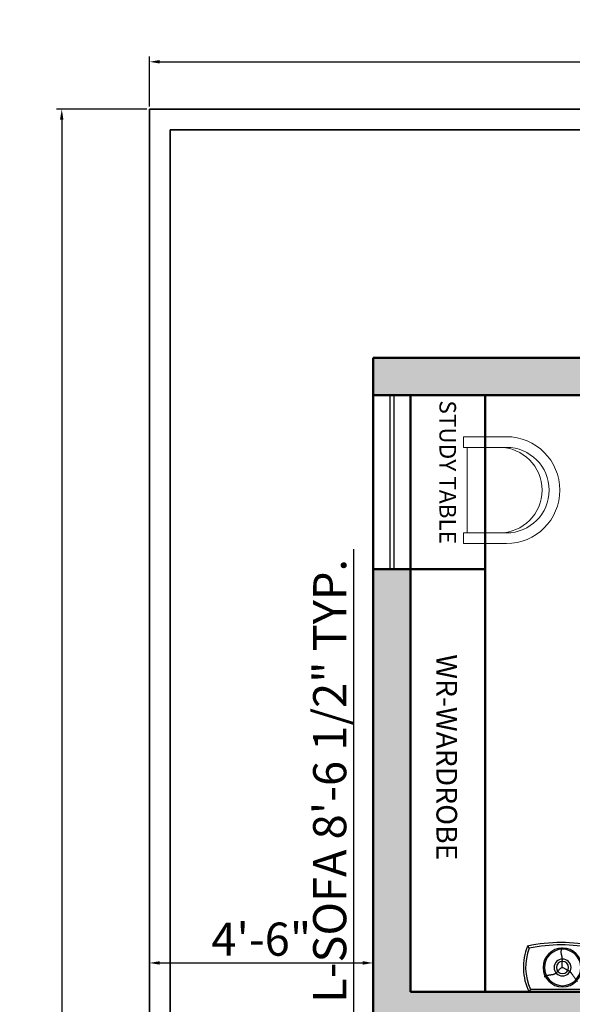
# Model space of a CAD drawing. Units: inches. Extents: x 3008 to 4088, y 1255 to 2137.
# Tile 26 of 30: x 3572 to 3705, y 1794 to 2031. Entities that reach past the tile are written whole.
import ezdxf

# ---------------------------------------------------------------- set-up
doc = ezdxf.new("R2010")
doc.units = ezdxf.units.IN
for name, color, linetype, lineweight in [('A-ANNO-DIMS', 2, 'Continuous', 18), ('A-ANNO-TEXT', 7, 'Continuous', 18), ('A-FURN', 8, 'Continuous', 18), ('A-GLAZ', 4, 'Continuous', 25), ('A-WALL', 7, 'Continuous', 50), ('A-WALL-PATT', 8, 'Continuous', 13), ('C-PROP', 1, 'Continuous', 35)]:
    doc.layers.add(name, color=color, linetype=linetype, lineweight=lineweight)
doc.layers.add('TEFRİŞ', color=11, linetype='Continuous')
doc.styles.get("Standard").update_dxf_attribs({"font": 'arial.ttf'})
doc.dimstyles.new('ISO-25', dxfattribs={"dimtxt": 8, "dimasz": 2.5, "dimexe": 1.25, "dimexo": 0.625, "dimtad": 1, "dimdec": 1, "dimlunit": 3, "dimtxsty": 'Standard', "dimcen": 2.5, "dimadec": 0, "dimazin": 0, "dimtfac": 1, "dimtdec": 1, "dimtmove": 0, "dimatfit": 3, "dimfxl": 1, "dimarcsym": 0})

# ---------------------------------------------------------------- blocks, each defined once
blk = doc.blocks.new('*D31')
at = {"layer": 'A-ANNO-DIMS', "color": 0, "lineweight": -2, "transparency": 16777216}
for p, q in [((3602.94, 2010.35), (3602.94, 2022.41)), ((4082.94, 2010.35), (4082.94, 2022.41)), ((3605.44, 2021.16), (4080.44, 2021.16))]:
    blk.add_line(p, q, dxfattribs=at)
at = {"layer": 'A-ANNO-DIMS', "color": 0, "transparency": 16777216}
for points in [[(3605.44, 2021.58), (3605.44, 2020.74), (3602.94, 2021.16)], [(4080.44, 2021.58), (4080.44, 2020.74), (4082.94, 2021.16)]]:
    blk.add_solid(points, dxfattribs=at)
at = {"layer": 'Defpoints', "color": 0, "transparency": 16777216}
for p in [(4082.94, 2021.16), (3602.94, 2009.72), (4082.94, 2009.72)]:
    blk.add_point(p, dxfattribs=at)
at = {"layer": 'A-ANNO-DIMS', "color": 0, "transparency": 16777216, "insert": (3842.94, 2025.87), "char_height": 8, "attachment_point": 5}
blk.add_mtext("40'", dxfattribs=at)
blk = doc.blocks.new('*D32')
at = {"layer": 'A-ANNO-DIMS', "color": 0, "lineweight": -2, "transparency": 16777216}
for p, q in [((3602.32, 2009.72), (3580.54, 2009.72)), ((3581.79, 2007.22), (3581.79, 1352.22)), ((3602.32, 1349.72), (3580.54, 1349.72))]:
    blk.add_line(p, q, dxfattribs=at)
at = {"layer": 'A-ANNO-DIMS', "color": 0, "transparency": 16777216}
for points in [[(3581.37, 2007.22), (3582.2, 2007.22), (3581.79, 2009.72)], [(3581.37, 1352.22), (3582.2, 1352.22), (3581.79, 1349.72)]]:
    blk.add_solid(points, dxfattribs=at)
at = {"layer": 'Defpoints', "color": 0, "transparency": 16777216}
for p in [(3602.94, 2009.72), (3581.79, 1349.72), (3602.94, 1349.72)]:
    blk.add_point(p, dxfattribs=at)
at = {"layer": 'A-ANNO-DIMS', "color": 0, "transparency": 16777216, "insert": (3577.09, 1679.72), "char_height": 8, "attachment_point": 5, "rotation": 90}
blk.add_mtext("55'", dxfattribs=at)
blk = doc.blocks.new('*D33')
at = {"layer": 'A-ANNO-DIMS', "color": 0, "lineweight": -2, "transparency": 16777216}
for p, q in [((3602.94, 1804.33), (3602.94, 1804.95)), ((3605.44, 1803.7), (3654.44, 1803.7)), ((3656.94, 1804.33), (3656.94, 1804.95))]:
    blk.add_line(p, q, dxfattribs=at)
at = {"layer": 'A-ANNO-DIMS', "color": 0, "transparency": 16777216}
for points in [[(3605.44, 1804.12), (3605.44, 1803.29), (3602.94, 1803.7)], [(3654.44, 1804.12), (3654.44, 1803.29), (3656.94, 1803.7)]]:
    blk.add_solid(points, dxfattribs=at)
at = {"layer": 'Defpoints', "color": 0, "transparency": 16777216}
for p in [(3602.94, 1803.7), (3656.94, 1803.7), (3656.94, 1803.7)]:
    blk.add_point(p, dxfattribs=at)
at = {"layer": 'A-ANNO-DIMS', "color": 0, "transparency": 16777216, "insert": (3629.94, 1808.41), "char_height": 8, "attachment_point": 5}
blk.add_mtext('4\'-6"', dxfattribs=at)
blk = doc.blocks.new('BED')
at = {"layer": 'TEFRİŞ'}
for p, q in [((2114.88, 1835.66), (2129.12, 1835.66)), ((2115.2, 1835.15), (2128.8, 1835.15)), ((2130.81, 1834.34), (2130.81, 1835.55)), ((2175.56, 1834.34), (2130.81, 1834.34)), ((2130.91, 1835.55), (2175.56, 1835.55)), ((2175, 1834.19), (2130.91, 1834.19)), ((2175.56, 1835.55), (2175.56, 1834.34)), ((2177.29, 1835.98), (2177.61, 1835.47)), ((2177.29, 1835.98), (2191.52, 1835.98)), ((2177.61, 1835.47), (2191.2, 1835.47)), ((2191.2, 1835.47), (2191.52, 1835.98)), ((2118.49, 1833.2), (2118.34, 1833.38)), ((2118.49, 1833.2), (2118.34, 1833.38)), ((2118.63, 1833.03), (2118.49, 1833.2)), ((2118.63, 1833.03), (2118.49, 1833.2)), ((2118.75, 1832.88), (2118.63, 1833.03)), ((2118.75, 1832.88), (2118.63, 1833.03)), ((2118.86, 1832.74), (2118.75, 1832.88)), ((2118.86, 1832.74), (2118.75, 1832.88)), ((2118.95, 1832.61), (2118.86, 1832.74)), ((2118.95, 1832.61), (2118.86, 1832.74)), ((2119.04, 1832.48), (2118.95, 1832.61)), ((2119.04, 1832.48), (2118.95, 1832.61)), ((2119.12, 1832.37), (2119.04, 1832.48)), ((2119.12, 1832.37), (2119.04, 1832.48)), ((2119.19, 1832.26), (2119.12, 1832.37)), ((2119.19, 1832.26), (2119.12, 1832.37)), ((2119.26, 1832.16), (2119.19, 1832.26)), ((2119.26, 1832.16), (2119.19, 1832.26)), ((2119.32, 1832.06), (2119.26, 1832.16)), ((2119.32, 1832.06), (2119.26, 1832.16)), ((2119.39, 1831.97), (2119.32, 1832.06)), ((2119.39, 1831.97), (2119.32, 1832.06)), ((2119.45, 1831.89), (2119.39, 1831.97)), ((2119.45, 1831.89), (2119.39, 1831.97)), ((2124.49, 1831.94), (2124.56, 1831.95)), ((2124.49, 1831.94), (2124.56, 1831.95)), ((2124.56, 1831.95), (2124.64, 1831.96)), ((2124.56, 1831.95), (2124.64, 1831.96)), ((2124.64, 1831.96), (2124.71, 1831.98)), ((2124.64, 1831.96), (2124.71, 1831.98)), ((2124.71, 1831.98), (2124.79, 1831.99)), ((2124.71, 1831.98), (2124.79, 1831.99)), ((2124.79, 1831.99), (2124.87, 1832.01)), ((2124.79, 1831.99), (2124.87, 1832.01)), ((2124.87, 1832.01), (2124.96, 1832.03)), ((2124.87, 1832.01), (2124.96, 1832.03)), ((2124.96, 1832.03), (2125.05, 1832.05)), ((2124.96, 1832.03), (2125.05, 1832.05)), ((2125.05, 1832.05), (2125.14, 1832.08)), ((2125.05, 1832.05), (2125.14, 1832.08)), ((2125.14, 1832.08), (2125.23, 1832.11)), ((2125.14, 1832.08), (2125.23, 1832.11)), ((2125.23, 1832.11), (2125.33, 1832.14)), ((2125.23, 1832.11), (2125.33, 1832.14)), ((2125.33, 1832.14), (2125.42, 1832.17)), ((2125.33, 1832.14), (2125.42, 1832.17)), ((2125.42, 1832.17), (2125.52, 1832.21)), ((2125.42, 1832.17), (2125.52, 1832.21)), ((2125.52, 1832.21), (2125.6, 1832.25)), ((2125.52, 1832.21), (2125.6, 1832.25)), ((2125.6, 1832.25), (2125.68, 1832.3)), ((2125.6, 1832.25), (2125.68, 1832.3)), ((2125.68, 1832.3), (2125.75, 1832.35)), ((2125.68, 1832.3), (2125.75, 1832.35)), ((2180.9, 1833.52), (2180.75, 1833.7)), ((2180.9, 1833.52), (2180.75, 1833.7)), ((2181.04, 1833.35), (2180.9, 1833.52)), ((2181.04, 1833.35), (2180.9, 1833.52)), ((2181.16, 1833.2), (2181.04, 1833.35)), ((2181.16, 1833.2), (2181.04, 1833.35)), ((2181.26, 1833.06), (2181.16, 1833.2)), ((2181.26, 1833.06), (2181.16, 1833.2)), ((2181.36, 1832.93), (2181.26, 1833.06)), ((2181.36, 1832.93), (2181.26, 1833.06)), ((2181.44, 1832.8), (2181.36, 1832.93)), ((2181.44, 1832.8), (2181.36, 1832.93)), ((2181.52, 1832.69), (2181.44, 1832.8)), ((2181.52, 1832.69), (2181.44, 1832.8)), ((2181.59, 1832.58), (2181.52, 1832.69)), ((2181.59, 1832.58), (2181.52, 1832.69)), ((2181.66, 1832.48), (2181.59, 1832.58)), ((2181.66, 1832.48), (2181.59, 1832.58)), ((2181.73, 1832.38), (2181.66, 1832.48)), ((2181.73, 1832.38), (2181.66, 1832.48)), ((2181.79, 1832.29), (2181.73, 1832.38)), ((2181.79, 1832.29), (2181.73, 1832.38)), ((2181.85, 1832.21), (2181.79, 1832.29)), ((2181.85, 1832.21), (2181.79, 1832.29)), ((2181.92, 1832.13), (2181.85, 1832.21)), ((2181.92, 1832.13), (2181.85, 1832.21)), ((2181.97, 1832.05), (2181.92, 1832.13)), ((2181.97, 1832.05), (2181.92, 1832.13)), ((2182.03, 1831.97), (2181.97, 1832.05)), ((2182.03, 1831.97), (2181.97, 1832.05)), ((2182.09, 1831.9), (2182.03, 1831.97)), ((2182.09, 1831.9), (2182.03, 1831.97)), ((2185.68, 1831.9), (2185.75, 1831.95)), ((2185.68, 1831.9), (2185.75, 1831.95)), ((2185.75, 1831.95), (2185.82, 1831.99)), ((2185.75, 1831.95), (2185.82, 1831.99)), ((2185.82, 1831.99), (2185.89, 1832.03)), ((2185.82, 1831.99), (2185.89, 1832.03)), ((2185.89, 1832.03), (2185.96, 1832.06)), ((2185.89, 1832.03), (2185.96, 1832.06)), ((2185.96, 1832.06), (2186.03, 1832.09)), ((2185.96, 1832.06), (2186.03, 1832.09)), ((2186.03, 1832.09), (2186.1, 1832.12)), ((2186.03, 1832.09), (2186.1, 1832.12)), ((2186.1, 1832.12), (2186.17, 1832.14)), ((2186.1, 1832.12), (2186.17, 1832.14)), ((2186.17, 1832.14), (2186.24, 1832.16)), ((2186.17, 1832.14), (2186.24, 1832.16)), ((2186.24, 1832.16), (2186.32, 1832.18)), ((2186.24, 1832.16), (2186.32, 1832.18)), ((2186.32, 1832.18), (2186.39, 1832.19)), ((2186.32, 1832.18), (2186.39, 1832.19)), ((2186.39, 1832.19), (2186.46, 1832.21)), ((2186.39, 1832.19), (2186.46, 1832.21)), ((2186.46, 1832.21), (2186.53, 1832.22)), ((2186.46, 1832.21), (2186.53, 1832.22)), ((2186.53, 1832.22), (2186.61, 1832.23)), ((2186.53, 1832.22), (2186.61, 1832.23)), ((2186.61, 1832.23), (2186.68, 1832.23)), ((2186.61, 1832.23), (2186.68, 1832.23)), ((2186.68, 1832.23), (2186.75, 1832.24)), ((2186.68, 1832.23), (2186.75, 1832.24)), ((2186.75, 1832.24), (2186.82, 1832.25)), ((2186.75, 1832.24), (2186.82, 1832.25)), ((2186.82, 1832.25), (2186.9, 1832.26)), ((2186.82, 1832.25), (2186.9, 1832.26)), ((2186.9, 1832.26), (2186.97, 1832.27)), ((2186.9, 1832.26), (2186.97, 1832.27)), ((2186.97, 1832.27), (2187.04, 1832.28)), ((2186.97, 1832.27), (2187.04, 1832.28)), ((2187.04, 1832.28), (2187.12, 1832.3)), ((2187.04, 1832.28), (2187.12, 1832.3)), ((2187.12, 1832.3), (2187.2, 1832.31)), ((2187.12, 1832.3), (2187.2, 1832.31)), ((2187.2, 1832.31), (2187.28, 1832.33)), ((2187.2, 1832.31), (2187.28, 1832.33)), ((2187.28, 1832.33), (2187.36, 1832.35)), ((2187.28, 1832.33), (2187.36, 1832.35)), ((2187.36, 1832.35), (2187.45, 1832.37)), ((2187.36, 1832.35), (2187.45, 1832.37)), ((2187.45, 1832.37), (2187.54, 1832.4)), ((2187.45, 1832.37), (2187.54, 1832.4)), ((2187.54, 1832.4), (2187.64, 1832.43)), ((2187.54, 1832.4), (2187.64, 1832.43)), ((2187.64, 1832.43), (2187.74, 1832.46)), ((2187.64, 1832.43), (2187.74, 1832.46)), ((2187.74, 1832.46), (2187.83, 1832.49)), ((2187.74, 1832.46), (2187.83, 1832.49)), ((2187.83, 1832.49), (2187.92, 1832.53)), ((2187.83, 1832.49), (2187.92, 1832.53)), ((2187.92, 1832.53), (2188.01, 1832.57)), ((2187.92, 1832.53), (2188.01, 1832.57)), ((2188.01, 1832.57), (2188.09, 1832.62)), ((2188.01, 1832.57), (2188.09, 1832.62)), ((2188.09, 1832.62), (2188.15, 1832.67)), ((2188.09, 1832.62), (2188.15, 1832.67)), ((2119.51, 1831.81), (2119.45, 1831.89)), ((2119.51, 1831.81), (2119.45, 1831.89)), ((2119.57, 1831.73), (2119.51, 1831.81)), ((2119.57, 1831.73), (2119.51, 1831.81)), ((2119.63, 1831.65), (2119.57, 1831.73)), ((2119.63, 1831.65), (2119.57, 1831.73)), ((2119.69, 1831.58), (2119.63, 1831.65)), ((2119.69, 1831.58), (2119.63, 1831.65)), ((2119.75, 1831.51), (2119.69, 1831.58)), ((2119.75, 1831.51), (2119.69, 1831.58)), ((2119.81, 1831.44), (2119.75, 1831.51)), ((2119.81, 1831.44), (2119.75, 1831.51)), ((2119.87, 1831.38), (2119.81, 1831.44)), ((2119.87, 1831.38), (2119.81, 1831.44)), ((2119.93, 1831.31), (2119.87, 1831.38)), ((2119.93, 1831.31), (2119.87, 1831.38)), ((2119.99, 1831.25), (2119.93, 1831.31)), ((2119.99, 1831.25), (2119.93, 1831.31)), ((2120.05, 1831.2), (2119.99, 1831.25)), ((2120.05, 1831.2), (2119.99, 1831.25)), ((2120.12, 1831.14), (2120.05, 1831.2)), ((2120.12, 1831.14), (2120.05, 1831.2)), ((2120.18, 1831.09), (2120.12, 1831.14)), ((2120.18, 1831.09), (2120.12, 1831.14)), ((2120.25, 1831.04), (2120.18, 1831.09)), ((2120.25, 1831.04), (2120.18, 1831.09)), ((2120.32, 1830.99), (2120.25, 1831.04)), ((2120.32, 1830.99), (2120.25, 1831.04)), ((2120.39, 1830.94), (2120.32, 1830.99)), ((2120.39, 1830.94), (2120.32, 1830.99)), ((2120.47, 1830.9), (2120.39, 1830.94)), ((2120.47, 1830.9), (2120.39, 1830.94)), ((2120.54, 1830.85), (2120.47, 1830.9)), ((2120.54, 1830.85), (2120.47, 1830.9)), ((2120.62, 1830.8), (2120.54, 1830.85)), ((2120.62, 1830.8), (2120.54, 1830.85)), ((2120.7, 1830.75), (2120.62, 1830.8)), ((2120.7, 1830.75), (2120.62, 1830.8)), ((2120.79, 1830.7), (2120.7, 1830.75)), ((2120.79, 1830.7), (2120.7, 1830.75)), ((2120.88, 1830.65), (2120.79, 1830.7)), ((2120.88, 1830.65), (2120.79, 1830.7)), ((2120.98, 1830.59), (2120.88, 1830.65)), ((2120.98, 1830.59), (2120.88, 1830.65)), ((2121.09, 1830.52), (2120.98, 1830.59)), ((2121.09, 1830.52), (2120.98, 1830.59)), ((2121.21, 1830.45), (2121.09, 1830.52)), ((2121.21, 1830.45), (2121.09, 1830.52)), ((2121.34, 1830.38), (2121.21, 1830.45)), ((2121.34, 1830.38), (2121.21, 1830.45)), ((2121.49, 1830.29), (2121.34, 1830.38)), ((2121.49, 1830.29), (2121.34, 1830.38)), ((2121.66, 1830.21), (2121.49, 1830.29)), ((2121.66, 1830.21), (2121.49, 1830.29)), ((2121.66, 1830.18), (2121.87, 1830.29)), ((2121.66, 1830.18), (2121.87, 1830.29)), ((2121.85, 1830.11), (2121.66, 1830.21)), ((2121.85, 1830.11), (2121.66, 1830.21)), ((2121.74, 1829.99), (2121.73, 1829.83)), ((2121.74, 1829.99), (2121.73, 1829.83)), ((2121.73, 1829.83), (2121.73, 1829.69)), ((2121.73, 1829.83), (2121.73, 1829.69)), ((2121.76, 1830.38), (2121.74, 1830.17)), ((2121.76, 1830.38), (2121.74, 1830.17)), ((2121.74, 1830.17), (2121.74, 1829.99)), ((2121.74, 1830.17), (2121.74, 1829.99)), ((2121.87, 1830.29), (2122.04, 1830.4)), ((2121.87, 1830.29), (2122.04, 1830.4)), ((2122.04, 1830.4), (2122.2, 1830.51)), ((2122.04, 1830.4), (2122.2, 1830.51)), ((2122.2, 1830.51), (2122.33, 1830.61)), ((2122.2, 1830.51), (2122.33, 1830.61)), ((2122.33, 1830.61), (2122.45, 1830.72)), ((2122.33, 1830.61), (2122.45, 1830.72)), ((2122.45, 1830.72), (2122.55, 1830.82)), ((2122.45, 1830.72), (2122.55, 1830.82)), ((2122.55, 1830.82), (2122.64, 1830.91)), ((2122.55, 1830.82), (2122.64, 1830.91)), ((2122.64, 1830.91), (2122.72, 1831.01)), ((2122.64, 1830.91), (2122.72, 1831.01)), ((2122.72, 1831.01), (2122.8, 1831.09)), ((2122.72, 1831.01), (2122.8, 1831.09)), ((2122.8, 1831.09), (2122.87, 1831.18)), ((2122.8, 1831.09), (2122.87, 1831.18)), ((2122.87, 1831.18), (2122.94, 1831.26)), ((2122.87, 1831.18), (2122.94, 1831.26)), ((2122.94, 1831.26), (2123.01, 1831.33)), ((2122.94, 1831.26), (2123.01, 1831.33)), ((2123.01, 1831.33), (2123.08, 1831.4)), ((2123.01, 1831.33), (2123.08, 1831.4)), ((2123.08, 1831.4), (2123.14, 1831.46)), ((2123.08, 1831.4), (2123.14, 1831.46)), ((2123.14, 1831.46), (2123.21, 1831.52)), ((2123.14, 1831.46), (2123.21, 1831.52)), ((2123.21, 1831.52), (2123.27, 1831.58)), ((2123.21, 1831.52), (2123.27, 1831.58)), ((2123.27, 1831.58), (2123.34, 1831.63)), ((2123.27, 1831.58), (2123.34, 1831.63)), ((2123.34, 1831.63), (2123.41, 1831.67)), ((2123.34, 1831.63), (2123.41, 1831.67)), ((2123.41, 1831.67), (2123.48, 1831.71)), ((2123.41, 1831.67), (2123.48, 1831.71)), ((2123.48, 1831.71), (2123.55, 1831.74)), ((2123.48, 1831.71), (2123.55, 1831.74)), ((2123.55, 1831.74), (2123.62, 1831.77)), ((2123.55, 1831.74), (2123.62, 1831.77)), ((2123.62, 1831.77), (2123.69, 1831.8)), ((2123.62, 1831.77), (2123.69, 1831.8)), ((2123.69, 1831.8), (2123.77, 1831.82)), ((2123.69, 1831.8), (2123.77, 1831.82)), ((2123.77, 1831.82), (2123.84, 1831.84)), ((2123.77, 1831.82), (2123.84, 1831.84)), ((2123.84, 1831.84), (2123.91, 1831.86)), ((2123.84, 1831.84), (2123.91, 1831.86)), ((2123.91, 1831.86), (2123.98, 1831.87)), ((2123.91, 1831.86), (2123.98, 1831.87)), ((2123.98, 1831.87), (2124.06, 1831.89)), ((2123.98, 1831.87), (2124.06, 1831.89)), ((2124.06, 1831.89), (2124.13, 1831.9)), ((2124.06, 1831.89), (2124.13, 1831.9)), ((2124.13, 1831.9), (2124.2, 1831.91)), ((2124.13, 1831.9), (2124.2, 1831.91)), ((2124.2, 1831.91), (2124.27, 1831.91)), ((2124.2, 1831.91), (2124.27, 1831.91)), ((2124.27, 1831.91), (2124.35, 1831.92)), ((2124.27, 1831.91), (2124.35, 1831.92)), ((2124.35, 1831.92), (2124.42, 1831.93)), ((2124.35, 1831.92), (2124.42, 1831.93)), ((2124.42, 1831.93), (2124.49, 1831.94)), ((2124.42, 1831.93), (2124.49, 1831.94)), ((2182.15, 1831.83), (2182.09, 1831.9)), ((2182.15, 1831.83), (2182.09, 1831.9)), ((2182.21, 1831.76), (2182.15, 1831.83)), ((2182.21, 1831.76), (2182.15, 1831.83)), ((2182.27, 1831.7), (2182.21, 1831.76)), ((2182.27, 1831.7), (2182.21, 1831.76)), ((2182.33, 1831.63), (2182.27, 1831.7)), ((2182.33, 1831.63), (2182.27, 1831.7)), ((2182.4, 1831.57), (2182.33, 1831.63)), ((2182.4, 1831.57), (2182.33, 1831.63)), ((2182.46, 1831.52), (2182.4, 1831.57)), ((2182.46, 1831.52), (2182.4, 1831.57)), ((2182.52, 1831.46), (2182.46, 1831.52)), ((2182.52, 1831.46), (2182.46, 1831.52)), ((2182.59, 1831.41), (2182.52, 1831.46)), ((2182.59, 1831.41), (2182.52, 1831.46)), ((2182.66, 1831.36), (2182.59, 1831.41)), ((2182.66, 1831.36), (2182.59, 1831.41)), ((2182.73, 1831.31), (2182.66, 1831.36)), ((2182.73, 1831.31), (2182.66, 1831.36)), ((2182.8, 1831.26), (2182.73, 1831.31)), ((2182.8, 1831.26), (2182.73, 1831.31)), ((2182.87, 1831.22), (2182.8, 1831.26)), ((2182.87, 1831.22), (2182.8, 1831.26)), ((2182.95, 1831.17), (2182.87, 1831.22)), ((2182.95, 1831.17), (2182.87, 1831.22)), ((2183.03, 1831.12), (2182.95, 1831.17)), ((2183.03, 1831.12), (2182.95, 1831.17)), ((2183.11, 1831.07), (2183.03, 1831.12)), ((2183.11, 1831.07), (2183.03, 1831.12)), ((2183.2, 1831.02), (2183.11, 1831.07)), ((2183.2, 1831.02), (2183.11, 1831.07)), ((2183.29, 1830.97), (2183.2, 1831.02)), ((2183.29, 1830.97), (2183.2, 1831.02)), ((2183.39, 1830.91), (2183.29, 1830.97)), ((2183.39, 1830.91), (2183.29, 1830.97)), ((2183.49, 1830.84), (2183.39, 1830.91)), ((2183.49, 1830.84), (2183.39, 1830.91)), ((2183.61, 1830.77), (2183.49, 1830.84)), ((2183.61, 1830.77), (2183.49, 1830.84)), ((2183.75, 1830.7), (2183.61, 1830.77)), ((2183.75, 1830.7), (2183.61, 1830.77)), ((2183.9, 1830.61), (2183.75, 1830.7)), ((2183.9, 1830.61), (2183.75, 1830.7)), ((2184.06, 1830.53), (2183.9, 1830.61)), ((2184.06, 1830.53), (2183.9, 1830.61)), ((2184.25, 1830.43), (2184.06, 1830.53)), ((2184.25, 1830.43), (2184.06, 1830.53)), ((2184.07, 1830.5), (2184.27, 1830.61)), ((2184.07, 1830.5), (2184.27, 1830.61)), ((2184.15, 1830.49), (2184.14, 1830.31)), ((2184.15, 1830.49), (2184.14, 1830.31)), ((2184.14, 1830.31), (2184.14, 1830.15)), ((2184.14, 1830.31), (2184.14, 1830.15)), ((2184.14, 1830.15), (2184.14, 1830.01)), ((2184.14, 1830.15), (2184.14, 1830.01)), ((2184.14, 1830.01), (2184.14, 1829.89)), ((2184.14, 1830.01), (2184.14, 1829.89)), ((2184.14, 1829.89), (2184.14, 1829.77)), ((2184.14, 1829.89), (2184.14, 1829.77)), ((2184.14, 1829.77), (2184.14, 1829.67)), ((2184.14, 1829.77), (2184.14, 1829.67)), ((2184.17, 1830.7), (2184.15, 1830.49)), ((2184.17, 1830.7), (2184.15, 1830.49)), ((2184.27, 1830.61), (2184.45, 1830.72)), ((2184.27, 1830.61), (2184.45, 1830.72)), ((2184.45, 1830.72), (2184.6, 1830.83)), ((2184.45, 1830.72), (2184.6, 1830.83)), ((2184.6, 1830.83), (2184.74, 1830.93)), ((2184.6, 1830.83), (2184.74, 1830.93)), ((2184.74, 1830.93), (2184.85, 1831.04)), ((2184.74, 1830.93), (2184.85, 1831.04)), ((2184.85, 1831.04), (2184.95, 1831.14)), ((2184.85, 1831.04), (2184.95, 1831.14)), ((2184.95, 1831.14), (2185.05, 1831.23)), ((2184.95, 1831.14), (2185.05, 1831.23)), ((2185.05, 1831.23), (2185.13, 1831.33)), ((2185.05, 1831.23), (2185.13, 1831.33)), ((2185.13, 1831.33), (2185.21, 1831.41)), ((2185.13, 1831.33), (2185.21, 1831.41)), ((2185.21, 1831.41), (2185.28, 1831.5)), ((2185.21, 1831.41), (2185.28, 1831.5)), ((2185.28, 1831.5), (2185.35, 1831.58)), ((2185.28, 1831.5), (2185.35, 1831.58)), ((2185.35, 1831.58), (2185.42, 1831.65)), ((2185.35, 1831.58), (2185.42, 1831.65)), ((2185.42, 1831.65), (2185.48, 1831.72)), ((2185.42, 1831.65), (2185.48, 1831.72)), ((2185.48, 1831.72), (2185.55, 1831.78)), ((2185.48, 1831.72), (2185.55, 1831.78)), ((2185.55, 1831.78), (2185.61, 1831.84)), ((2185.55, 1831.78), (2185.61, 1831.84)), ((2185.61, 1831.84), (2185.68, 1831.9)), ((2185.61, 1831.84), (2185.68, 1831.9)), ((2121.73, 1829.69), (2121.73, 1829.57)), ((2121.73, 1829.69), (2121.73, 1829.57)), ((2121.73, 1829.57), (2121.73, 1829.45)), ((2121.73, 1829.57), (2121.73, 1829.45)), ((2121.73, 1829.45), (2121.74, 1829.35)), ((2121.73, 1829.45), (2121.74, 1829.35)), ((2121.74, 1828.89), (2121.73, 1828.8)), ((2121.74, 1828.89), (2121.73, 1828.8)), ((2121.73, 1828.8), (2121.73, 1828.72)), ((2121.73, 1828.8), (2121.73, 1828.72)), ((2121.73, 1828.72), (2121.73, 1828.64)), ((2121.73, 1828.72), (2121.73, 1828.64)), ((2121.73, 1828.64), (2121.73, 1828.56)), ((2121.73, 1828.64), (2121.73, 1828.56)), ((2121.73, 1828.56), (2121.73, 1828.48)), ((2121.73, 1828.56), (2121.73, 1828.48)), ((2121.73, 1828.48), (2121.73, 1828.4)), ((2121.73, 1828.48), (2121.73, 1828.4)), ((2121.73, 1828.4), (2121.73, 1828.33)), ((2121.73, 1828.4), (2121.73, 1828.33)), ((2121.73, 1828.33), (2121.74, 1828.25)), ((2121.73, 1828.33), (2121.74, 1828.25)), ((2121.74, 1829.35), (2121.74, 1829.25)), ((2121.74, 1829.35), (2121.74, 1829.25)), ((2121.74, 1829.25), (2121.74, 1829.16)), ((2121.74, 1829.25), (2121.74, 1829.16)), ((2121.74, 1829.16), (2121.74, 1829.06)), ((2121.74, 1829.16), (2121.74, 1829.06)), ((2121.74, 1829.06), (2121.74, 1828.97)), ((2121.74, 1829.06), (2121.74, 1828.97)), ((2121.74, 1828.97), (2121.74, 1828.89)), ((2121.74, 1828.97), (2121.74, 1828.89)), ((2121.74, 1828.25), (2121.75, 1828.18)), ((2121.74, 1828.25), (2121.75, 1828.18)), ((2121.75, 1828.18), (2121.75, 1828.1)), ((2121.75, 1828.18), (2121.75, 1828.1)), ((2121.75, 1828.1), (2121.76, 1828.03)), ((2121.75, 1828.1), (2121.76, 1828.03)), ((2121.76, 1828.03), (2121.78, 1827.95)), ((2121.76, 1828.03), (2121.78, 1827.95)), ((2121.78, 1827.95), (2121.79, 1827.88)), ((2121.78, 1827.95), (2121.79, 1827.88)), ((2121.79, 1827.88), (2121.8, 1827.8)), ((2121.79, 1827.88), (2121.8, 1827.8)), ((2121.8, 1827.8), (2121.82, 1827.72)), ((2121.8, 1827.8), (2121.82, 1827.72)), ((2121.82, 1827.72), (2121.84, 1827.65)), ((2121.82, 1827.72), (2121.84, 1827.65)), ((2121.84, 1827.65), (2121.85, 1827.57)), ((2121.84, 1827.65), (2121.85, 1827.57)), ((2184.14, 1829.04), (2184.13, 1828.96)), ((2184.14, 1829.04), (2184.13, 1828.96)), ((2184.13, 1828.96), (2184.13, 1828.88)), ((2184.13, 1828.96), (2184.13, 1828.88)), ((2184.13, 1828.88), (2184.13, 1828.8)), ((2184.13, 1828.88), (2184.13, 1828.8)), ((2184.13, 1828.8), (2184.14, 1828.72)), ((2184.13, 1828.8), (2184.14, 1828.72)), ((2184.14, 1829.67), (2184.15, 1829.57)), ((2184.14, 1829.67), (2184.15, 1829.57)), ((2184.15, 1829.38), (2184.14, 1829.29)), ((2184.15, 1829.38), (2184.14, 1829.29)), ((2184.14, 1829.29), (2184.14, 1829.21)), ((2184.14, 1829.29), (2184.14, 1829.21)), ((2184.14, 1829.21), (2184.14, 1829.12)), ((2184.14, 1829.21), (2184.14, 1829.12)), ((2184.14, 1829.12), (2184.14, 1829.04)), ((2184.14, 1829.12), (2184.14, 1829.04)), ((2184.14, 1828.72), (2184.14, 1828.65)), ((2184.14, 1828.72), (2184.14, 1828.65)), ((2184.14, 1828.65), (2184.15, 1828.57)), ((2184.14, 1828.65), (2184.15, 1828.57)), ((2184.15, 1829.57), (2184.15, 1829.48)), ((2184.15, 1829.57), (2184.15, 1829.48)), ((2184.15, 1829.48), (2184.15, 1829.38)), ((2184.15, 1829.48), (2184.15, 1829.38)), ((2184.15, 1828.57), (2184.15, 1828.5)), ((2184.15, 1828.57), (2184.15, 1828.5)), ((2184.15, 1828.5), (2184.16, 1828.42)), ((2184.15, 1828.5), (2184.16, 1828.42)), ((2184.16, 1828.42), (2184.17, 1828.35)), ((2184.16, 1828.42), (2184.17, 1828.35)), ((2184.17, 1828.35), (2184.18, 1828.27)), ((2184.17, 1828.35), (2184.18, 1828.27)), ((2184.18, 1828.27), (2184.19, 1828.2)), ((2184.18, 1828.27), (2184.19, 1828.2)), ((2184.19, 1828.2), (2184.21, 1828.12)), ((2184.19, 1828.2), (2184.21, 1828.12)), ((2184.21, 1828.12), (2184.22, 1828.04)), ((2184.21, 1828.12), (2184.22, 1828.04)), ((2184.22, 1828.04), (2184.24, 1827.97)), ((2184.22, 1828.04), (2184.24, 1827.97)), ((2184.24, 1827.97), (2184.26, 1827.89)), ((2184.24, 1827.97), (2184.26, 1827.89)), ((2184.26, 1827.89), (2184.28, 1827.81)), ((2184.26, 1827.89), (2184.28, 1827.81)), ((2184.28, 1827.81), (2184.3, 1827.73)), ((2184.28, 1827.81), (2184.3, 1827.73)), ((2184.3, 1827.73), (2184.32, 1827.65)), ((2184.3, 1827.73), (2184.32, 1827.65)), ((2184.32, 1827.65), (2184.34, 1827.58)), ((2184.32, 1827.65), (2184.34, 1827.58)), ((2184.34, 1827.58), (2184.36, 1827.5)), ((2184.34, 1827.58), (2184.36, 1827.5)), ((2121.78, 1825.93), (2121.74, 1825.8)), ((2121.78, 1825.93), (2121.74, 1825.8)), ((2121.83, 1826.06), (2121.78, 1825.93)), ((2121.83, 1826.06), (2121.78, 1825.93)), ((2121.87, 1826.19), (2121.83, 1826.06)), ((2121.87, 1826.19), (2121.83, 1826.06)), ((2121.85, 1827.57), (2121.87, 1827.49)), ((2121.85, 1827.57), (2121.87, 1827.49)), ((2121.87, 1827.49), (2121.89, 1827.41)), ((2121.87, 1827.49), (2121.89, 1827.41)), ((2121.91, 1826.31), (2121.87, 1826.19)), ((2121.91, 1826.31), (2121.87, 1826.19)), ((2121.89, 1827.41), (2121.91, 1827.33)), ((2121.89, 1827.41), (2121.91, 1827.33)), ((2121.91, 1827.33), (2121.93, 1827.26)), ((2121.91, 1827.33), (2121.93, 1827.26)), ((2121.95, 1826.42), (2121.91, 1826.31)), ((2121.95, 1826.42), (2121.91, 1826.31)), ((2121.93, 1827.26), (2121.95, 1827.18)), ((2121.93, 1827.26), (2121.95, 1827.18)), ((2121.95, 1827.18), (2121.97, 1827.09)), ((2121.95, 1827.18), (2121.97, 1827.09)), ((2121.97, 1826.54), (2121.95, 1826.42)), ((2121.97, 1826.54), (2121.95, 1826.42)), ((2121.97, 1827.09), (2121.99, 1827.01)), ((2121.97, 1827.09), (2121.99, 1827.01)), ((2121.99, 1826.64), (2121.97, 1826.54)), ((2121.99, 1826.64), (2121.97, 1826.54)), ((2121.99, 1827.01), (2122, 1826.93)), ((2121.99, 1827.01), (2122, 1826.93)), ((2122, 1826.74), (2121.99, 1826.64)), ((2122, 1826.74), (2121.99, 1826.64)), ((2122, 1826.93), (2122.01, 1826.84)), ((2122, 1826.93), (2122.01, 1826.84)), ((2122.01, 1826.84), (2122, 1826.74)), ((2122.01, 1826.84), (2122, 1826.74)), ((2129.46, 1825.49), (2129.09, 1825.93)), ((2176.94, 1825.81), (2177.31, 1826.25)), ((2184.19, 1826.25), (2184.14, 1826.12)), ((2184.19, 1826.25), (2184.14, 1826.12)), ((2184.23, 1826.38), (2184.19, 1826.25)), ((2184.23, 1826.38), (2184.19, 1826.25)), ((2184.28, 1826.51), (2184.23, 1826.38)), ((2184.28, 1826.51), (2184.23, 1826.38)), ((2184.32, 1826.63), (2184.28, 1826.51)), ((2184.32, 1826.63), (2184.28, 1826.51)), ((2184.35, 1826.74), (2184.32, 1826.63)), ((2184.35, 1826.74), (2184.32, 1826.63)), ((2184.38, 1826.86), (2184.35, 1826.74)), ((2184.38, 1826.86), (2184.35, 1826.74)), ((2184.36, 1827.5), (2184.38, 1827.41)), ((2184.36, 1827.5), (2184.38, 1827.41)), ((2184.38, 1827.41), (2184.4, 1827.33)), ((2184.38, 1827.41), (2184.4, 1827.33)), ((2184.4, 1826.96), (2184.38, 1826.86)), ((2184.4, 1826.96), (2184.38, 1826.86)), ((2184.4, 1827.33), (2184.41, 1827.25)), ((2184.4, 1827.33), (2184.41, 1827.25)), ((2184.41, 1827.06), (2184.4, 1826.96)), ((2184.41, 1827.06), (2184.4, 1826.96)), ((2184.41, 1827.25), (2184.41, 1827.16)), ((2184.41, 1827.25), (2184.41, 1827.16)), ((2184.41, 1827.16), (2184.41, 1827.06)), ((2184.41, 1827.16), (2184.41, 1827.06)), ((2191.87, 1825.81), (2191.5, 1826.25)), ((2174.77, 1819.77), (2130.6, 1795.83)), ((2174.77, 1820.53), (2130.76, 1800.91)), ((2140.43, 1818.69), (2131.53, 1818.69)), ((2141.43, 1817.4), (2131.53, 1817.4)), ((2149.62, 1817.4), (2145.88, 1817.4)), ((2167.36, 1817.4), (2154.77, 1817.4)), ((2157.71, 1818.69), (2156.77, 1818.69)), ((2170.41, 1818.69), (2164.92, 1818.69)), ((2175, 1776.57), (2130.11, 1776.57)), ((2138.52, 1775.41), (2167.39, 1775.41))]:
    blk.add_line(p, q, dxfattribs=at)
for centre, radius, start, end in [((2126, 1830.19), 12.39, 153.8162, 202.314), ((2126, 1830.19), 11.88, 155.3335, 201.0157), ((2118, 1830.19), 11.88, 338.9843, 24.6665), ((2118, 1830.19), 12.39, 337.686, 26.1838), ((2188.4, 1830.51), 12.39, 153.8162, 202.314), ((2188.4, 1830.51), 11.88, 155.3335, 201.0157), ((2180.41, 1830.51), 11.88, 338.9843, 24.6665), ((2180.41, 1830.51), 12.39, 337.686, 26.1838), ((2122, 1861.35), 36.63, 258.2443, 281.7557), ((2122, 1861.35), 36.12, 258.6773, 281.3227), ((2184.41, 1861.67), 36.63, 258.2443, 281.7557), ((2184.41, 1861.67), 36.12, 258.6773, 281.3227)]:
    blk.add_arc(centre, radius, start, end, dxfattribs=at)
at = {"layer": 'TEFRİŞ', "extrusion": (0, 0, -1)}
for centre, major_axis, ratio, start_param, end_param in [((2121.68, 1830.24), (-3.05, -3.05), 1, 3.926991, 10.210176), ((2121.68, 1830.24), (2.86, -2.86), 1, 5.497787, 11.780972), ((2121.68, 1830.24), (2.86, -2.86), 1, 5.497787, 11.780972), ((2206.14, 1830.73), (-52.86, -52.86), 1, 0.767743, 0.83177), ((2138.85, 1803.05), (-22.1, 22.1), 1, 0.544604, 1.006234), ((2154.12, 1796.61), (-26.46, 26.46), 1, 0.596409, 0.940188), ((2168.35, 1789.27), (-1.33, 44.62), 0.875277, -0.163954, 0.163954), ((2167.6, 1797.72), (-0.51, 36.47), 0.865194, -0.185965, 0.185965), ((2184.09, 1830.56), (-3.05, -3.05), 1, 3.926991, 10.210176), ((2184.09, 1830.56), (2.86, -2.86), 1, 5.497787, 11.780972), ((2184.09, 1830.56), (2.86, -2.86), 1, 5.497787, 11.780972), ((2121.68, 1830.24), (1.33, -1.33), 1, 5.497787, 11.780972), ((2121.68, 1830.24), (1.33, -1.33), 1, 5.497787, 11.780972), ((2139.43, 1773.84), (-42.35, 42.35), 1, 0.646251, 0.896949), ((2154.7, 1828.89), (-15.68, 15.68), 1, -1.00675, -0.580436), ((2181.61, 1828.44), (-34.39, 34.39), 1, -0.888486, -0.672463), ((2164.51, 1832.79), (-13.41, 13.41), 1, -0.974476, -0.730892), ((2127.6, 1828.81), (-13.23, 13.23), 1, 2.100388, 2.328052), ((2155, 1761.9), (-50.65, -50.65), 1, 2.239512, 2.426533), ((2172.01, 1828.66), (-17.93, 17.93), 1, -0.753394, -0.598744), ((2128.44, 1832.96), (-13.26, -13.26), 1, 3.889049, 4.127298), ((2183.72, 1833.22), (-17, 17), 1, -0.967105, -0.749712), ((2134, 1828.8), (-18.62, 18.62), 1, 2.173461, 2.355043), ((2199.2, 1828.45), (-27.06, -27.06), 1, 0.770625, 0.917228), ((2087.32, 1833.96), (-52.37, 52.37), 1, 2.358049, 2.431787), ((2164.15, 1828.7), (-6.99, 6.99), 1, 1.789136, 2.946702), ((2156.76, 1828.98), (-11.9, -11.9), 1, 3.646453, 4.226155), ((2099.77, 1830.73), (-52.86, 52.86), 1, 2.311571, 2.373849), ((2184.09, 1830.56), (1.33, -1.33), 1, 5.497787, 11.780972), ((2184.09, 1830.56), (1.33, -1.33), 1, 5.497787, 11.780972), ((2184.09, 1830.56), (0.952, -0.952), 1, 5.497787, 11.780972), ((2184.09, 1830.56), (0.952, -0.952), 1, 5.497787, 11.780972), ((2121.68, 1830.24), (0.952, -0.952), 1, 5.497787, 11.780972), ((2121.68, 1830.24), (0.952, -0.952), 1, 5.497787, 11.780972), ((2159.55, 1823.33), (-5.81, 5.81), 1, -0.516587, 0.256776), ((2154.84, 1827.75), (-1.93, 1.93), 1, 0.997904, 1.977819), ((2166.67, 1824.96), (-2.93, 3.91), 0.760601, -0.723751, 0.723751), ((2675.38, 1815.09), (-384.79, -384.79), 1, 0.80103, 0.811711), ((2147.44, 1824.41), (-3.36, -3.36), 1, 1.11934, 2.270556), ((2145.66, 1827.01), (-1.62, 1.62), 1, 1.310976, 2.284591), ((2172, 1826.44), (-11.23, 11.23), 1, -1.332486, -0.624868), ((2158.82, 1823.55), (-3.74, -3.74), 1, 1.730792, 3.47045), ((2141.71, 1819.83), (-11.86, 11.86), 1, 1.850844, 2.42862), ((2157.83, 1821.53), (-4.47, 4.47), 1, 0.576679, 2.021689), ((2153.88, 1825.05), (-9.22, 9.22), 1, 1.994956, 2.818753), ((1630.53, 1815.09), (-384.79, 384.79), 1, 2.329881, 2.340562), ((2140.05, 1819.86), (-5.1, 5.1), 1, 0.238357, 1.390139), ((2139.42, 1820.79), (-4.21, -4.21), 1, 1.82161, 3.349145), ((2148.15, 1825.25), (-7.14, -7.14), 1, 6.061986, 7.190757), ((2154.93, 1828.48), (-11.96, 11.96), 1, -1.530302, -0.934407), ((2127.37, 1815.76), (-10.68, 10.68), 1, 1.657204, 1.779381), ((2160.6, 1825.98), (-9.68, -9.68), 1, 0.009196, 0.886853), ((2148.35, 1820.65), (-4.63, -4.63), 1, 2.117602, 3.020837), ((2147.86, 1820.64), (-4.48, 4.48), 1, 0.665914, 1.867503), ((2170.68, 1829.67), (-16.79, 16.79), 1, -1.354718, -0.902276), ((2146.08, 1822.57), (-10.5, 10.5), 1, -0.951783, -0.716225), ((2132.43, 1774.09), (-35.41, -35.41), 1, 2.362911, 2.464592), ((2140.17, 1862.96), (-27.99, 27.99), 1, 3.983025, 4.107469), ((2165.73, 1860.69), (-26.41, -26.41), 1, 5.306413, 5.463767), ((2199.62, 1529.47), (-209.2, 209.2), 1, 0.675361, 0.697001), ((2159.82, 1822.57), (-10.5, -10.5), 1, 3.857817, 4.093375), ((2127.37, 1815.76), (-10.68, 10.68), 1, 1.94252, 2.248924), ((2111.06, 1818.12), (-14.48, 14.48), 1, 2.258605, 2.412359), ((2141.33, 1830.48), (-9.55, -9.55), 1, 4.941413, 5.601673), ((2150.79, 1825.18), (-6, 6), 1, 3.032122, 4.026148), ((2159.02, 1834.9), (-3.04, 16.53), 0.830169, 2.822117, 3.461068), ((2194.85, 1818.12), (-14.48, 14.48), 1, -0.841563, -0.687809), ((2169.92, 1815.01), (-27.2, -27.2), 1, 0.734393, 0.836404), ((2135.98, 1815.01), (-27.2, -27.2), 1, 3.875985, 3.977996), ((2098.24, 1811.68), (-23.54, -23.54), 1, 3.885834, 4.043401), ((2207.66, 1811.68), (-23.54, -23.54), 1, 0.668988, 0.826555), ((2189.03, 1803.74), (-40.91, -40.91), 1, 0.789771, 0.855756), ((2116.87, 1803.74), (-40.91, 40.91), 1, 2.285836, 2.351822), ((2122.14, 1803.63), (-6.39, -6.39), 1, 3.886359, 4.265474), ((2222.76, 1798.77), (-34.16, -34.16), 1, 0.743488, 0.893627), ((2135.02, 1798.41), (-3.45, 3.45), 1, -0.831635, -0.314979), ((2135.48, 1798), (-3.77, -3.77), 1, 0.329385, 0.820948), ((2127.76, 1790.23), (-1, 12.37), 0.296708, 1.141067, 2.000525), ((2148.06, 1790.38), (-0.75, 67.37), 0.394952, 1.480524, 1.661068), ((2118.49, 1784.2), (-9.24, -9.24), 1, 3.839645, 4.088086), ((2182.27, 1782.99), (-5.52, -5.52), 1, 0.671703, 0.993321), ((2162.12, 1778.86), (-21.85, 21.85), 1, -0.78611, -0.680117), ((2143.78, 1778.86), (-21.85, 21.85), 1, 2.250913, 2.356906), ((2132.72, 1775.92), (-1.91, -1.91), 1, 0.284117, 1.557111), ((2129.83, 1778.8), (-0.986, 0.986), 1, 2.330985, 3.163296), ((2176.08, 1778.8), (-0.986, 0.986), 1, 4.690686, 5.522997), ((2173.18, 1775.92), (-1.91, -1.91), 1, 3.155278, 4.428271), ((2134.73, 1774.06), (-0.964, -0.964), 1, 1.381176, 2.701227), ((2136.75, 1781.14), (-4.24, 4.24), 1, 3.62713, 4.188813), ((2169.16, 1781.14), (-4.24, 4.24), 1, 3.665169, 4.226852), ((2171.17, 1774.06), (-0.964, -0.964), 1, 2.011162, 3.331212), ((2131.79, 1775.28), (-1.11, 1.11), 1, 3.629269, 5.067473), ((2130.83, 1777), (-2.49, -2.49), 1, 4.590984, 5.084038), ((2175.07, 1777), (-2.49, 2.49), 1, 4.34074, 4.833793), ((2174.12, 1775.28), (-1.11, 1.11), 1, 2.786508, 4.224712)]:
    blk.add_ellipse(centre, major_axis=major_axis, ratio=ratio, start_param=start_param, end_param=end_param, dxfattribs=at)
blk = doc.blocks.new('12PSTG07')
at = {"color": 0, "linetype": 'ByBlock'}
for p, q in [((0, 15), (-12, 15)), ((0, 12), (0, 15)), ((-12, 12), (0, 12)), ((-1, -12), (-1, 12)), ((-12, -12), (0, -12)), ((0, -12), (0, -15)), ((0, -15), (-12, -15))]:
    blk.add_line(p, q, dxfattribs=at)
for centre, radius in [((-12, 0), 15), ((-12, 0), 12), ((-10, 0), 12)]:
    blk.add_arc(centre, radius, 90, 270, dxfattribs=at)
blk = doc.blocks.new('*D57')
at = {"layer": 'A-ANNO-DIMS', "color": 0, "lineweight": -2, "transparency": 16777216}
for p, q in [((3652.25, 1789.25), (3652.25, 1903.53)), ((3666.98, 1789.25), (3651, 1789.25)), ((3652.25, 1689.39), (3652.25, 1786.75)), ((3666.98, 1686.89), (3651, 1686.89))]:
    blk.add_line(p, q, dxfattribs=at)
at = {"layer": 'A-ANNO-DIMS', "color": 0, "transparency": 16777216}
for points in [[(3651.83, 1786.75), (3652.67, 1786.75), (3652.25, 1789.25)], [(3651.83, 1689.39), (3652.67, 1689.39), (3652.25, 1686.89)]]:
    blk.add_solid(points, dxfattribs=at)
at = {"layer": 'Defpoints', "color": 0, "transparency": 16777216}
for p in [(3652.25, 1789.25), (3667.61, 1789.25), (3667.61, 1686.89)]:
    blk.add_point(p, dxfattribs=at)
at = {"layer": 'A-ANNO-DIMS', "color": 0, "transparency": 16777216, "insert": (3647.49, 1847.64), "char_height": 8, "attachment_point": 5, "rotation": 90}
blk.add_mtext('L-SOFA 8\'-6 1/2" TYP.', dxfattribs=at)

msp = doc.modelspace()

# ---------------------------------------------------------------- hatches: boundary and pattern name
at = {"layer": 'A-WALL-PATT'}
h = msp.add_hatch(color=256, dxfattribs=at)
h.dxf.hatch_style = 1
h.paths.add_polyline_path([(3665.94, 1631.72), (3656.94, 1631.72), (3656.94, 1546.72), (3665.94, 1546.72)])
h.paths.add_polyline_path([(3851.94, 1619.72), (3701.94, 1619.72), (3701.94, 1610.72), (3788.94, 1610.72), (3788.94, 1469.72), (3809.94, 1469.72), (3809.94, 1478.72), (3797.94, 1478.72), (3797.94, 1550.72), (3815.94, 1550.72), (3815.94, 1556.72), (3797.94, 1556.72), (3797.94, 1610.72), (3845.94, 1610.72), (3845.94, 1586.72), (3851.94, 1586.72)])
h.paths.add_polyline_path([(4028.94, 1631.72), (4019.94, 1631.72), (4019.94, 1619.72), (3887.94, 1619.72), (3887.94, 1610.72), (4019.94, 1610.72), (4019.94, 1577.72), (4028.94, 1577.72)])
h.paths.add_polyline_path([(3875.94, 1478.72), (3851.94, 1478.72), (3851.94, 1556.72), (3845.94, 1556.72), (3845.94, 1526.72), (3845.94, 1478.72), (3833.94, 1478.72), (3833.94, 1469.72), (3875.94, 1469.72)])
h.paths.add_polyline_path([(3959.94, 1478.72), (3917.94, 1478.72), (3917.94, 1469.72), (3959.94, 1469.72)])
h.paths.add_polyline_path([(4028.94, 1511.72), (4019.94, 1511.72), (4019.94, 1478.72), (4001.94, 1478.72), (4001.94, 1469.72), (4028.94, 1469.72)])
h.paths.add_polyline_path([(4028.94, 1699.22), (4019.94, 1699.22), (4019.94, 1673.72), (3893.94, 1673.72), (3893.94, 1649.72), (3899.94, 1649.72), (3899.94, 1667.72), (4019.94, 1667.72), (4019.94, 1655.72), (4028.94, 1655.72)])
h.paths.add_polyline_path([(4028.94, 1847.72), (4019.94, 1847.72), (4019.94, 1796.72), (3863.94, 1796.72), (3863.94, 1790.72), (4019.94, 1790.72), (4019.94, 1765.22), (4028.94, 1765.22)])
h.paths.add_polyline_path([(3815.94, 1796.72), (3779.94, 1796.72), (3665.94, 1796.72), (3665.94, 1898.72), (3656.94, 1898.72), (3656.94, 1673.72), (3665.94, 1673.72), (3665.94, 1790.72), (3815.94, 1790.72)])
h.paths.add_polyline_path([(3755.94, 1949.72), (3656.94, 1949.72), (3656.94, 1940.72), (3665.94, 1940.72), (3755.94, 1940.72)])
h.paths.add_polyline_path([(3827.94, 1949.72), (3797.94, 1949.72), (3797.94, 1940.72), (3809.94, 1940.72), (3809.94, 1874.72), (3815.94, 1874.72), (3815.94, 1940.72), (3827.94, 1940.72)])
h.paths.add_polyline_path([(3953.94, 1949.72), (3851.94, 1949.72), (3851.94, 1940.72), (3863.94, 1940.72), (3863.94, 1844.72), (3809.94, 1844.72), (3809.94, 1832.72), (3815.94, 1832.72), (3815.94, 1838.72), (3863.94, 1838.72), (3869.94, 1838.72), (3869.94, 1940.72), (3953.94, 1940.72)])
h.paths.add_polyline_path([(4028.94, 1949.72), (3995.94, 1949.72), (3995.94, 1940.72), (4019.94, 1940.72), (4019.94, 1889.72), (4028.94, 1889.72)])

# ---------------------------------------------------------------- linework, layer by layer
at = {"layer": 'A-GLAZ'}
for p, q in [((3660.94, 1940.72), (3660.94, 1898.72)), ((3660.94, 1940.72), (3660.94, 1898.72)), ((3661.94, 1940.72), (3661.94, 1898.72))]:
    msp.add_line(p, q, dxfattribs=at)
at = {"layer": 'A-WALL'}
for p, q in [((3656.94, 1949.72), (4028.94, 1949.72)), ((3656.94, 1546.72), (3656.94, 1949.72)), ((3656.94, 1940.72), (3665.94, 1940.72)), ((3665.94, 1940.72), (3809.94, 1940.72)), ((3665.94, 1796.72), (3665.94, 1940.72)), ((3683.94, 1796.72), (3683.94, 1940.72)), ((3656.94, 1898.72), (3683.94, 1898.72)), ((3665.94, 1796.72), (3815.94, 1796.72))]:
    msp.add_line(p, q, dxfattribs=at)
at = {"layer": 'C-PROP'}
for p, q in [((3602.94, 2009.72), (4082.94, 2009.72)), ((3602.94, 1349.72), (3602.94, 2009.72)), ((3607.94, 2004.72), (4077.94, 2004.72)), ((3607.94, 1354.72), (3607.94, 2004.72))]:
    msp.add_line(p, q, dxfattribs=at)

# ---------------------------------------------------------------- block references
at = {"layer": 'A-FURN', "rotation": 180}
for name, p, xscale, yscale, zscale in [('12PSTG07', (3678.78, 1917.79), 0.8597921787217941, 0.8597921787217941, 0.8597921787217941), ('BED', (6076.48, 3792.2), 1.086875874800008, 1.086875874800008, 1.086875874800008)]:
    msp.add_blockref(name, p, dxfattribs=dict(at, xscale=xscale, yscale=yscale, zscale=zscale))

# ---------------------------------------------------------------- texts
at = {"layer": 'A-ANNO-TEXT', "attachment_point": 1, "rotation": 270}
for s, insert, char_height in [('{\\fTimes New Roman|b0|i0|c0|p18;STUDY TABLE}', (3676.94, 1939.46), 4), ('{\\fTimes New Roman|b0|i0|c0|p18;WR-WARDROBE}', (3677.21, 1878.2), 5)]:
    msp.add_mtext_dynamic_manual_height_columns(s, width=105.6127, gutter_width=12.5, heights=[0], dxfattribs=dict(at, insert=insert, char_height=char_height))

# ---------------------------------------------------------------- dimensions: what is measured, and where the dimension line sits
at = {"layer": 'A-ANNO-DIMS'}
for base, p1, p2, picture, middle in [((4082.94, 2021.16), (3602.94, 2009.72), (4082.94, 2009.72), '*D31', (3842.94, 2025.87)), ((3656.94, 1803.7), (3602.94, 1803.7), (3656.94, 1803.7), '*D33', (3629.94, 1808.41))]:
    dim = msp.add_linear_dim(base=base, p1=p1, p2=p2, dimstyle='ISO-25', override={"dimclrd": 0, "dimclre": 0, "dimclrt": 0}, dxfattribs=at)
    dim.commit()
    dim.dimension.update_dxf_attribs({"geometry": picture, "text_midpoint": middle})
dim = msp.add_linear_dim(base=(3581.79, 1349.72), p1=(3602.94, 2009.72), p2=(3602.94, 1349.72), angle=90, dimstyle='ISO-25', override={"dimclrd": 0, "dimclre": 0, "dimclrt": 0}, dxfattribs=at)
dim.commit()
dim.dimension.update_dxf_attribs({"geometry": '*D32', "text_midpoint": (3577.09, 1679.72)})
dim = msp.add_linear_dim(base=(3652.25, 1789.25), p1=(3667.61, 1686.89), p2=(3667.61, 1789.25), angle=90, text='L-SOFA <> TYP.', dimstyle='ISO-25', override={"dimdec": 1, "dimrnd": 0, "dimzin": 1, "dimlunit": 4, "dimfrac": 2}, dxfattribs=at)
dim.commit()
dim.dimension.update_dxf_attribs({"geometry": '*D57', "text_midpoint": (3647.49, 1847.64)})

doc.saveas('drawing.dxf')
